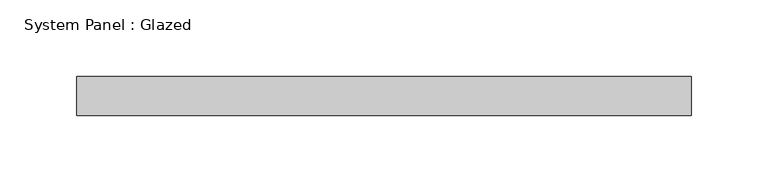
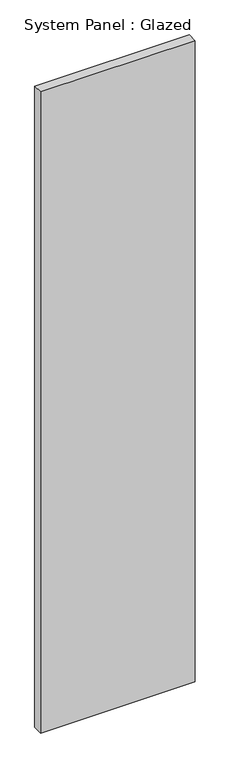
"""IFC4 building model written with IfcOpenShell, lengths in millimetres: plate geometry, System Panel : Glazed."""

from ifc_helpers import new_model, si_unit, origin, origin_with_axes, place, context, project, spatial, polyline, outline, extrude, source, transform, mapped, element, save


def system_panel_glazed_d030299f(model_context):
    return source(origin(), model_context, "Body", "SweptSolid", [
        extrude(outline(polyline([(200.025, 19.05), (-200.025, 19.05), (-200.025, 44.45), (200.025, 44.45), (200.025, 19.05)])), origin_with_axes(), (0.0, 0.0, 1.0), 1752.6),
    ])


if __name__ == "__main__":
    model = new_model("IFC4")
    model_context = context("Model", 3, world=origin())
    ifc_project = project(units=[si_unit("LENGTHUNIT", "METRE", prefix="MILLI")], contexts=[model_context])
    site = spatial("IfcSite", under=ifc_project)
    building = spatial("IfcBuilding", under=site)
    placement = place(None, origin())
    system_panel_glazed_shape = system_panel_glazed_d030299f(model_context)
    element("IfcPlate", 1, ObjectType="System Panel : Glazed", at=placement, inside=building, context=model_context, shape_type="MappedRepresentation", body=[
        mapped(system_panel_glazed_shape, transform((0.0, 0.0, 0.0), x_axis=(1.0, 0.0, 0.0), y_axis=(0.0, 1.0, 0.0), z_axis=(0.0, 0.0, 1.0))),
    ])
    save(model, "model.ifc")

# Revit data of these elements
# Type "System Panel : Glazed"
#   Construction Type Id = "GSP4R"
#   Analytic Construction = "1/8 in Pilkington single glazing"
#   Visual Light Transmittance = 0.9
#   Solar Heat Gain Coefficient = 0.86
#   Heat Transfer Coefficient (U) = 1.18115 BTU/(h·ft²·°F)
#   Define Thermal Properties by = 1
# Element 1 (IfcPlate, "System Panel : Glazed")
#   Materials on its faces: "Glass"
# Materials
#   "Glass": class "Glass", colour RGB 0 128 192, transparency 0.75, Description = "Soda Lime Glass", Cost = 0
